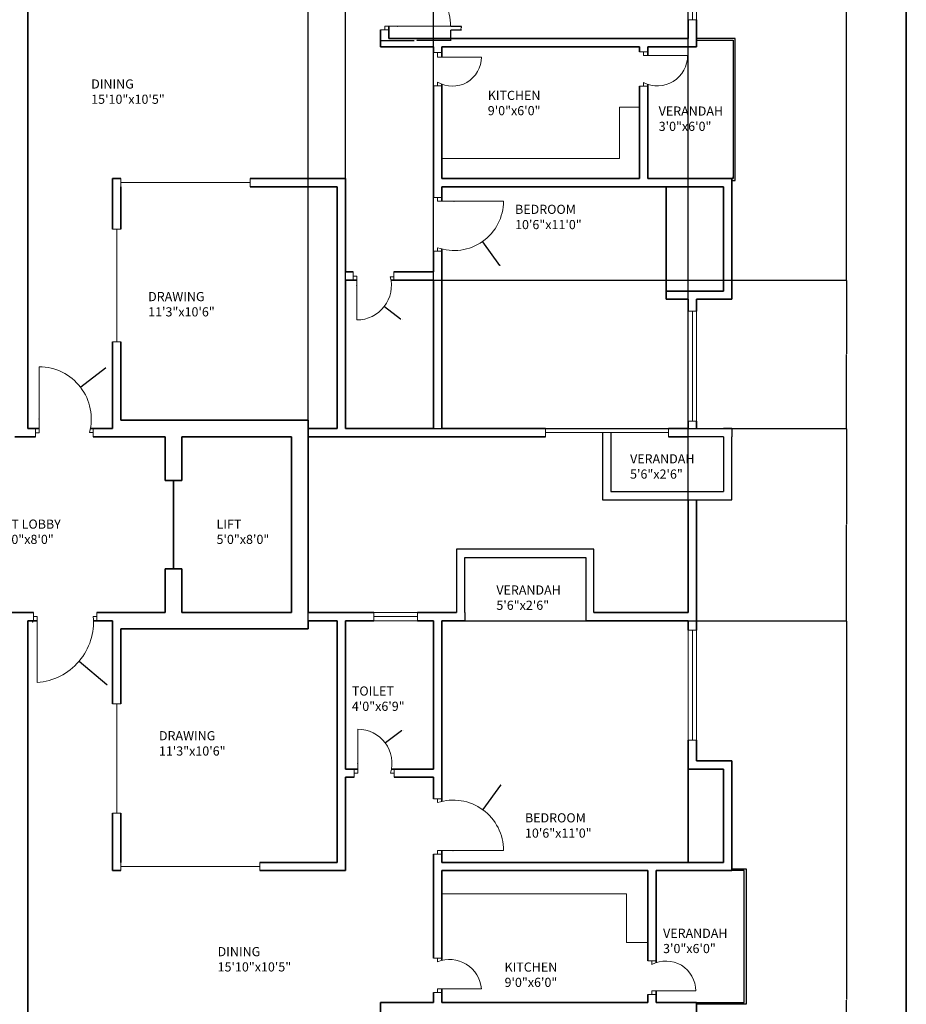
# Model space of a CAD drawing. Units: inches. Extents: x 2154 to 3131, y 1384 to 2688.
# Tile 4 of 5: x 2647 to 3131, y 1828 to 2365. Entities that reach past the tile are written whole.
import ezdxf

# ---------------------------------------------------------------- set-up
doc = ezdxf.new("R2010")
doc.units = ezdxf.units.IN
for name, color, linetype, lineweight in [('A-ANNO-DIMS', 2, 'Continuous', 18), ('A-ANNO-TTLB', 7, 'Continuous', 35), ('A-AREA-IDEN', 7, 'Continuous', 18), ('A-DOOR', 31, 'Continuous', 18), ('A-FLOR-BALC', 130, 'Continuous', 25), ('A-FLOR-EVTR', 7, 'Continuous', 35), ('A-FLOR-FIXT', 8, 'Continuous', 18), ('A-GLAZ', 130, 'Continuous', 18), ('A-WALL', 7, 'Continuous', 35)]:
    doc.layers.add(name, color=color, linetype=linetype, lineweight=lineweight)
doc.styles.get("Standard").update_dxf_attribs({"font": 'arial.ttf'})
doc.dimstyles.get("Standard").update_dxf_attribs({"dimtxt": 0.18, "dimasz": 0.18, "dimexe": 0.18, "dimexo": 0.0625, "dimgap": 0.09, "dimtad": 0, "dimtih": 1, "dimtoh": 1, "dimdec": 4, "dimzin": 0, "dimdsep": 46, "dimtxsty": 'Standard', "dimcen": 0.09, "dimadec": 0, "dimazin": 0, "dimtfac": 1, "dimtdec": 4, "dimtofl": 0, "dimtmove": 0, "dimatfit": 3, "dimfxl": 1, "dimtolj": 1, "dimtzin": 0, "dimarcsym": 0})

# ---------------------------------------------------------------- blocks, each defined once
blk = doc.blocks.new('DOOR-LEAF-24-JAMB-A')
for p, q in [((0, 2.25), (0, 26.25)), ((2, 2.25), (0, 2.25)), ((2, 4.5), (2, 0)), ((2, 0), (2, 2.25))]:
    blk.add_line(p, q)
blk = doc.blocks.new('DOOR-LEAF-36-JAMB-A')
for p, q in [((2, 2.25), (2, 38.25)), ((0, 4.5), (0, 0)), ((0, 0), (0, 2.25)), ((0, 2.25), (2, 2.25))]:
    blk.add_line(p, q)
blk = doc.blocks.new('DOOR-LEAF-24-JAMB-B')
for p, q in [((0, 2), (4.5, 2)), ((4.5, 2), (2.25, 2)), ((2.25, 2), (2.25, 0)), ((2.25, 0), (26.25, 0))]:
    blk.add_line(p, q)
blk = doc.blocks.new('DOOR-LEAF-36-JAMB-B')
for p, q in [((2.25, 0), (2.25, 2)), ((2.25, 2), (38.25, 2)), ((0, 0), (4.5, 0)), ((4.5, 0), (2.25, 0))]:
    blk.add_line(p, q)
blk = doc.blocks.new('WIN-60')
for p, q in [((2.25, 60), (0, 60)), ((0, 60), (4.5, 60)), ((0, 60), (0, 0)), ((2.25, 0), (2.25, 60)), ((4.5, 60), (4.5, 0)), ((0, 0), (4.5, 0)), ((4.5, 0), (2.25, 0))]:
    blk.add_line(p, q)
blk = doc.blocks.new('WIN-24-FRAME-B')
for p, q in [((0, 0), (0, 4.5)), ((0, 4.5), (24, 4.5)), ((24, 2.25), (0, 2.25)), ((0, 2.25), (0, 0)), ((24, 4.5), (24, 0)), ((24, 0), (24, 2.25)), ((24, 0), (0, 0))]:
    blk.add_line(p, q)
blk = doc.blocks.new('*D14')
at = {"layer": 'A-ANNO-DIMS', "color": 0, "lineweight": -2, "transparency": 16777216}
for p, q in [((2844.16, 2359.75), (2844.16, 2353.89)), ((2882.41, 2359.75), (2882.41, 2353.89)), ((2844.34, 2354.07), (2862.56, 2354.07)), ((2882.23, 2354.07), (2864, 2354.07))]:
    blk.add_line(p, q, dxfattribs=at)
at = {"layer": 'A-ANNO-DIMS', "color": 0, "transparency": 16777216}
for points in [[(2844.34, 2354.1), (2844.34, 2354.04), (2844.16, 2354.07)], [(2882.23, 2354.1), (2882.23, 2354.04), (2882.41, 2354.07)]]:
    blk.add_solid(points, dxfattribs=at)
at = {"layer": 'Defpoints', "color": 0, "transparency": 16777216}
for p in [(2844.16, 2359.81), (2882.41, 2359.81), (2882.41, 2354.07)]:
    blk.add_point(p, dxfattribs=at)
at = {"layer": 'A-ANNO-DIMS', "color": 0, "transparency": 16777216, "insert": (2863.28, 2354.07), "char_height": 0.18, "attachment_point": 5}
blk.add_mtext('\\A1;D4 38 TYP.', dxfattribs=at)
blk = doc.blocks.new('*D15')
at = {"layer": 'A-ANNO-DIMS', "color": 0, "lineweight": -2, "transparency": 16777216}
for p, q in [((2882.47, 2361.81), (2888.32, 2361.81)), ((2888.14, 2361.63), (2888.14, 2360.99)), ((2882.47, 2359.81), (2888.32, 2359.81)), ((2888.14, 2359.99), (2888.14, 2360.63))]:
    blk.add_line(p, q, dxfattribs=at)
at = {"layer": 'A-ANNO-DIMS', "color": 0, "transparency": 16777216}
for points in [[(2888.11, 2361.63), (2888.17, 2361.63), (2888.14, 2361.81)], [(2888.11, 2359.99), (2888.17, 2359.99), (2888.14, 2359.81)]]:
    blk.add_solid(points, dxfattribs=at)
at = {"layer": 'Defpoints', "color": 0, "transparency": 16777216}
for p in [(2882.41, 2361.81), (2888.14, 2361.81), (2882.41, 2359.81)]:
    blk.add_point(p, dxfattribs=at)
at = {"layer": 'A-ANNO-DIMS', "color": 0, "transparency": 16777216, "insert": (2888.14, 2360.81), "char_height": 0.18, "attachment_point": 5}
blk.add_mtext('\\A1;2 TYP.', dxfattribs=at)
blk = doc.blocks.new('*D27')
at = {"layer": 'A-ANNO-DIMS', "color": 0, "lineweight": -2, "transparency": 16777216}
for p, q in [((2804.6, 2037.24), (2804.6, 2635.76)), ((2804.78, 2635.58), (2907.91, 2635.58)), ((3011.98, 2635.58), (2908.84, 2635.58)), ((3012.16, 2041.74), (3012.16, 2635.76))]:
    blk.add_line(p, q, dxfattribs=at)
at = {"layer": 'A-ANNO-DIMS', "color": 0, "transparency": 16777216}
for points in [[(2804.78, 2635.61), (2804.78, 2635.55), (2804.6, 2635.58)], [(3011.98, 2635.61), (3011.98, 2635.55), (3012.16, 2635.58)]]:
    blk.add_solid(points, dxfattribs=at)
at = {"layer": 'Defpoints', "color": 0, "transparency": 16777216}
for p in [(3012.16, 2635.58), (3012.16, 2041.68), (2804.6, 2037.18)]:
    blk.add_point(p, dxfattribs=at)
at = {"layer": 'A-ANNO-DIMS', "color": 0, "transparency": 16777216, "insert": (2908.38, 2635.58), "char_height": 0.18, "attachment_point": 5}
blk.add_mtext('\\A1;207.56', dxfattribs=at)
blk = doc.blocks.new('*D30')
at = {"layer": 'A-ANNO-DIMS', "color": 0, "lineweight": -2, "transparency": 16777216}
for p, q in [((3012.22, 2037.18), (3098.74, 2037.18)), ((3098.56, 2037), (3098.56, 1830.36)), ((3098.56, 1623.36), (3098.56, 1830)), ((3016.72, 1623.18), (3098.74, 1623.18))]:
    blk.add_line(p, q, dxfattribs=at)
at = {"layer": 'A-ANNO-DIMS', "color": 0, "transparency": 16777216}
for points in [[(3098.53, 2037), (3098.59, 2037), (3098.56, 2037.18)], [(3098.53, 1623.36), (3098.59, 1623.36), (3098.56, 1623.18)]]:
    blk.add_solid(points, dxfattribs=at)
at = {"layer": 'Defpoints', "color": 0, "transparency": 16777216}
for p in [(3012.16, 2037.18), (3098.56, 2037.18), (3016.66, 1623.18)]:
    blk.add_point(p, dxfattribs=at)
at = {"layer": 'A-ANNO-DIMS', "color": 0, "transparency": 16777216, "insert": (3098.56, 1830.18), "char_height": 0.18, "attachment_point": 5}
blk.add_mtext('\\A1;414', dxfattribs=at)
blk = doc.blocks.new('*D31')
at = {"layer": 'A-ANNO-DIMS', "color": 0, "lineweight": -2, "transparency": 16777216}
for p, q in [((3016.72, 2142.21), (3098.74, 2142.21)), ((3098.56, 2142.03), (3098.56, 2089.87)), ((3098.56, 2037.36), (3098.56, 2089.51)), ((3012.22, 2037.18), (3098.74, 2037.18))]:
    blk.add_line(p, q, dxfattribs=at)
at = {"layer": 'A-ANNO-DIMS', "color": 0, "transparency": 16777216}
for points in [[(3098.53, 2142.03), (3098.59, 2142.03), (3098.56, 2142.21)], [(3098.53, 2037.36), (3098.59, 2037.36), (3098.56, 2037.18)]]:
    blk.add_solid(points, dxfattribs=at)
at = {"layer": 'Defpoints', "color": 0, "transparency": 16777216}
for p in [(3016.66, 2142.21), (3098.56, 2142.21), (3012.16, 2037.18)]:
    blk.add_point(p, dxfattribs=at)
at = {"layer": 'A-ANNO-DIMS', "color": 0, "transparency": 16777216, "insert": (3098.56, 2089.69), "char_height": 0.18, "attachment_point": 5}
blk.add_mtext('\\A1;105.03', dxfattribs=at)
blk = doc.blocks.new('*D32')
at = {"layer": 'A-ANNO-DIMS', "color": 0, "lineweight": -2, "transparency": 16777216}
for p, q in [((2873.1, 2223.18), (3098.74, 2223.18)), ((3098.56, 2223), (3098.56, 2182.86)), ((3098.56, 2142.36), (3098.56, 2182.49)), ((2873.1, 2142.18), (3098.74, 2142.18))]:
    blk.add_line(p, q, dxfattribs=at)
at = {"layer": 'A-ANNO-DIMS', "color": 0, "transparency": 16777216}
for points in [[(3098.53, 2223), (3098.59, 2223), (3098.56, 2223.18)], [(3098.53, 2142.36), (3098.59, 2142.36), (3098.56, 2142.18)]]:
    blk.add_solid(points, dxfattribs=at)
at = {"layer": 'Defpoints', "color": 0, "transparency": 16777216}
for p in [(2873.04, 2223.18), (3098.56, 2223.18), (2873.04, 2142.18)]:
    blk.add_point(p, dxfattribs=at)
at = {"layer": 'A-ANNO-DIMS', "color": 0, "transparency": 16777216, "insert": (3098.56, 2182.68), "char_height": 0.18, "attachment_point": 5}
blk.add_mtext('\\A1;81', dxfattribs=at)
blk = doc.blocks.new('*D33')
at = {"layer": 'A-ANNO-DIMS', "color": 0, "lineweight": -2, "transparency": 16777216}
for p, q in [((3016.72, 2562.18), (3098.74, 2562.18)), ((3098.56, 2562), (3098.56, 2392.86)), ((3098.56, 2223.36), (3098.56, 2392.49)), ((2873.1, 2223.18), (3098.74, 2223.18))]:
    blk.add_line(p, q, dxfattribs=at)
at = {"layer": 'A-ANNO-DIMS', "color": 0, "transparency": 16777216}
for points in [[(3098.53, 2562), (3098.59, 2562), (3098.56, 2562.18)], [(3098.53, 2223.36), (3098.59, 2223.36), (3098.56, 2223.18)]]:
    blk.add_solid(points, dxfattribs=at)
at = {"layer": 'Defpoints', "color": 0, "transparency": 16777216}
for p in [(3016.66, 2562.18), (3098.56, 2562.18), (2873.04, 2223.18)]:
    blk.add_point(p, dxfattribs=at)
at = {"layer": 'A-ANNO-DIMS', "color": 0, "transparency": 16777216, "insert": (3098.56, 2392.68), "char_height": 0.18, "attachment_point": 5}
blk.add_mtext('\\A1;339', dxfattribs=at)
blk = doc.blocks.new('*D34')
at = {"layer": 'A-ANNO-DIMS', "color": 0, "lineweight": -2, "transparency": 16777216}
for p, q in [((2825.04, 2142.24), (2825.04, 2635.76)), ((2825.22, 2635.58), (2848.81, 2635.58)), ((2872.86, 2635.58), (2849.26, 2635.58)), ((2873.04, 2142.24), (2873.04, 2635.76))]:
    blk.add_line(p, q, dxfattribs=at)
at = {"layer": 'A-ANNO-DIMS', "color": 0, "transparency": 16777216}
for points in [[(2825.22, 2635.61), (2825.22, 2635.55), (2825.04, 2635.58)], [(2872.86, 2635.61), (2872.86, 2635.55), (2873.04, 2635.58)]]:
    blk.add_solid(points, dxfattribs=at)
at = {"layer": 'Defpoints', "color": 0, "transparency": 16777216}
for p in [(2873.04, 2635.58), (2825.04, 2142.18), (2873.04, 2142.18)]:
    blk.add_point(p, dxfattribs=at)
at = {"layer": 'A-ANNO-DIMS', "color": 0, "transparency": 16777216, "insert": (2849.04, 2635.58), "char_height": 0.18, "attachment_point": 5}
blk.add_mtext('\\A1;48', dxfattribs=at)
blk = doc.blocks.new('*D35')
at = {"layer": 'A-ANNO-DIMS', "color": 0, "lineweight": -2, "transparency": 16777216}
for p, q in [((2654.17, 2036.55), (2654.35, 2036.55)), ((2654.26, 2036.46), (2654.26, 2036.64)), ((2694.7, 2002.08), (2679.67, 2014.89)), ((2694.88, 2002.08), (2694.7, 2002.08))]:
    blk.add_line(p, q, dxfattribs=at)
at = {"layer": 'A-ANNO-DIMS', "color": 0, "transparency": 16777216}
blk.add_solid([(2679.69, 2014.91), (2679.65, 2014.87), (2679.53, 2015.01)], dxfattribs=at)
at = {"layer": 'Defpoints', "color": 0, "transparency": 16777216}
for p in [(2654.26, 2036.55), (2679.53, 2015.01)]:
    blk.add_point(p, dxfattribs=at)
at = {"layer": 'A-ANNO-DIMS', "color": 0, "transparency": 16777216, "insert": (2695.43, 2002.08), "char_height": 0.18, "attachment_point": 5}
blk.add_mtext('\\A1;R33.214', dxfattribs=at)
blk = doc.blocks.new('*D40')
at = {"layer": 'A-ANNO-DIMS', "color": 0, "lineweight": -2, "transparency": 16777216}
for p, q in [((2882.03, 2398.4), (2871.38, 2384.82)), ((2882.21, 2398.4), (2882.03, 2398.4)), ((2853.25, 2361.81), (2853.43, 2361.81)), ((2853.34, 2361.72), (2853.34, 2361.9))]:
    blk.add_line(p, q, dxfattribs=at)
at = {"layer": 'A-ANNO-DIMS', "color": 0, "transparency": 16777216}
blk.add_solid([(2871.36, 2384.84), (2871.41, 2384.8), (2871.27, 2384.68)], dxfattribs=at)
at = {"layer": 'Defpoints', "color": 0, "transparency": 16777216}
for p in [(2871.27, 2384.68), (2853.34, 2361.81)]:
    blk.add_point(p, dxfattribs=at)
at = {"layer": 'A-ANNO-DIMS', "color": 0, "transparency": 16777216, "insert": (2882.69, 2398.4), "char_height": 0.18, "attachment_point": 5}
blk.add_mtext('\\A1;R29.06', dxfattribs=at)
blk = doc.blocks.new('*D43')
at = {"layer": 'A-ANNO-DIMS', "color": 0, "lineweight": -2, "transparency": 16777216}
for p, q in [((2693.94, 2175.05), (2680.52, 2164.77)), ((2694.12, 2175.05), (2693.94, 2175.05)), ((2657.68, 2147.34), (2657.86, 2147.34)), ((2657.77, 2147.25), (2657.77, 2147.43))]:
    blk.add_line(p, q, dxfattribs=at)
at = {"layer": 'A-ANNO-DIMS', "color": 0, "transparency": 16777216}
blk.add_solid([(2680.5, 2164.79), (2680.54, 2164.75), (2680.38, 2164.66)], dxfattribs=at)
at = {"layer": 'Defpoints', "color": 0, "transparency": 16777216}
for p in [(2680.38, 2164.66), (2657.77, 2147.34)]:
    blk.add_point(p, dxfattribs=at)
at = {"layer": 'A-ANNO-DIMS', "color": 0, "transparency": 16777216, "insert": (2694.6, 2175.05), "char_height": 0.18, "attachment_point": 5}
blk.add_mtext('\\A1;R28.48', dxfattribs=at)
blk = doc.blocks.new('*D47')
at = {"layer": 'A-ANNO-DIMS', "color": 0, "lineweight": -2, "transparency": 16777216}
for p, q in [((2909.69, 1947.29), (2900.06, 1934.08)), ((2909.87, 1947.29), (2909.69, 1947.29)), ((2883.64, 1911.66), (2883.82, 1911.66)), ((2883.73, 1911.57), (2883.73, 1911.75))]:
    blk.add_line(p, q, dxfattribs=at)
at = {"layer": 'A-ANNO-DIMS', "color": 0, "transparency": 16777216}
blk.add_solid([(2900.04, 1934.1), (2900.09, 1934.06), (2899.96, 1933.93)], dxfattribs=at)
at = {"layer": 'Defpoints', "color": 0, "transparency": 16777216}
for p in [(2899.96, 1933.93), (2883.73, 1911.66)]:
    blk.add_point(p, dxfattribs=at)
at = {"layer": 'A-ANNO-DIMS', "color": 0, "transparency": 16777216, "insert": (2910.42, 1947.29), "char_height": 0.18, "attachment_point": 5}
blk.add_mtext('\\A1;R27.553', dxfattribs=at)
blk = doc.blocks.new('*D49')
at = {"layer": 'A-ANNO-DIMS', "color": 0, "lineweight": -2, "transparency": 16777216}
for p, q in [((2884.2, 2266.37), (2884.38, 2266.37)), ((2884.29, 2266.28), (2884.29, 2266.46)), ((2909.23, 2231.09), (2899.98, 2244.17)), ((2909.41, 2231.09), (2909.23, 2231.09))]:
    blk.add_line(p, q, dxfattribs=at)
at = {"layer": 'A-ANNO-DIMS', "color": 0, "transparency": 16777216}
blk.add_solid([(2900, 2244.19), (2899.95, 2244.16), (2899.88, 2244.32)], dxfattribs=at)
at = {"layer": 'Defpoints', "color": 0, "transparency": 16777216}
for p in [(2884.29, 2266.37), (2899.88, 2244.32)]:
    blk.add_point(p, dxfattribs=at)
at = {"layer": 'A-ANNO-DIMS', "color": 0, "transparency": 16777216, "insert": (2909.71, 2231.09), "char_height": 0.18, "attachment_point": 5}
blk.add_mtext('\\A1;R27', dxfattribs=at)
blk = doc.blocks.new('*D59')
at = {"layer": 'A-ANNO-DIMS', "color": 0, "lineweight": -2, "transparency": 16777216}
for p, q in [((2831.18, 2220.22), (2831.36, 2220.22)), ((2831.27, 2220.13), (2831.27, 2220.31)), ((2855.11, 2201.9), (2846.31, 2208.66)), ((2855.29, 2201.9), (2855.11, 2201.9))]:
    blk.add_line(p, q, dxfattribs=at)
at = {"layer": 'A-ANNO-DIMS', "color": 0, "transparency": 16777216}
blk.add_solid([(2846.33, 2208.68), (2846.29, 2208.63), (2846.17, 2208.77)], dxfattribs=at)
at = {"layer": 'Defpoints', "color": 0, "transparency": 16777216}
for p in [(2831.27, 2220.22), (2846.17, 2208.77)]:
    blk.add_point(p, dxfattribs=at)
at = {"layer": 'A-ANNO-DIMS', "color": 0, "transparency": 16777216, "insert": (2855.84, 2201.9), "char_height": 0.18, "attachment_point": 5}
blk.add_mtext('\\A1;R18.793', dxfattribs=at)
blk = doc.blocks.new('*D60')
at = {"layer": 'A-ANNO-DIMS', "color": 0, "lineweight": -2, "transparency": 16777216}
for p, q in [((2855.66, 1977.05), (2846.84, 1970.51)), ((2855.84, 1977.05), (2855.66, 1977.05)), ((2831.67, 1959.34), (2831.85, 1959.34)), ((2831.76, 1959.25), (2831.76, 1959.43))]:
    blk.add_line(p, q, dxfattribs=at)
at = {"layer": 'A-ANNO-DIMS', "color": 0, "transparency": 16777216}
blk.add_solid([(2846.82, 1970.54), (2846.86, 1970.49), (2846.7, 1970.4)], dxfattribs=at)
at = {"layer": 'Defpoints', "color": 0, "transparency": 16777216}
for p in [(2846.7, 1970.4), (2831.76, 1959.34)]:
    blk.add_point(p, dxfattribs=at)
at = {"layer": 'A-ANNO-DIMS', "color": 0, "transparency": 16777216, "insert": (2856.32, 1977.05), "char_height": 0.18, "attachment_point": 5}
blk.add_mtext('\\A1;R18.59', dxfattribs=at)

msp = doc.modelspace()

# ---------------------------------------------------------------- linework, layer by layer
at = {"layer": 'A-ANNO-TTLB'}
msp.add_lwpolyline([(2154.1953, 2688.4009), (3131.1627, 2688.4009), (3131.1627, 1383.7377), (2154.1953, 1383.7377)], close=True, dxfattribs=at)
at = {"layer": 'A-DOOR'}
for p, q in [((2873.0368, 2347.5192), (2877.5368, 2347.5192)), ((2877.5368, 2347.5192), (2875.2868, 2347.5192)), ((2875.2868, 2347.5192), (2875.2868, 2347.0346)), ((2875.2868, 2347.0346), (2875.2868, 2345.0346)), ((2875.2868, 2345.0346), (2899.2868, 2345.0346)), ((2873.0368, 2329.273), (2877.5368, 2329.273)), ((2875.2868, 2329.273), (2875.2868, 2331.273)), ((2877.5368, 2329.273), (2875.2868, 2329.273)), ((2985.5368, 2329.0685), (2990.0368, 2329.0685)), ((2987.7868, 2329.0685), (2987.7868, 2331.0685)), ((2990.0368, 2329.0685), (2987.7868, 2329.0685)), ((2873.0368, 2238.9097), (2877.5368, 2238.9097)), ((2875.2868, 2238.9097), (2875.2868, 2240.9097)), ((2877.5368, 2238.9097), (2875.2868, 2238.9097)), ((2851.4271, 2226.9339), (2851.4271, 2227.6767)), ((2851.4271, 2227.6767), (2851.4271, 2225.0553)), ((2851.4271, 2223.1767), (2851.4271, 2226.9339)), ((2851.4271, 2225.0553), (2849.4271, 2225.0553)), ((2657.7665, 2139.8207), (2657.7665, 2175.8207)), ((2655.7665, 2142.1767), (2655.7665, 2137.6767)), ((2687.2664, 2142.1767), (2687.2664, 2137.6767)), ((2655.7665, 2137.6767), (2655.7665, 2139.8207)), ((2655.7665, 2139.8207), (2655.7665, 2139.8207)), ((2655.7665, 2139.8207), (2657.7665, 2139.8207)), ((2687.2664, 2139.9267), (2685.2664, 2139.9267)), ((2687.2664, 2137.6767), (2687.2664, 2139.9267)), ((2689.347, 2039.4267), (2687.347, 2039.4267)), ((2689.347, 2037.1767), (2689.347, 2041.6767)), ((2689.347, 2041.6767), (2689.347, 2039.4267)), ((2851.5443, 1953.9267), (2849.5443, 1953.9267)), ((2851.5443, 1956.1767), (2851.5443, 1951.6767)), ((2851.5443, 1951.6767), (2851.5443, 1953.9267)), ((2873.0368, 1939.8885), (2877.5368, 1939.8885)), ((2877.5368, 1939.8885), (2875.2868, 1939.8885)), ((2875.2868, 1939.8885), (2875.2868, 1937.8885)), ((2873.0368, 1852.9368), (2877.5368, 1852.9368)), ((2877.5368, 1852.9368), (2875.2868, 1852.9368)), ((2875.2868, 1852.9368), (2875.2868, 1850.9368)), ((2994.5368, 1851.4405), (2990.0368, 1851.4405)), ((2990.0368, 1851.4405), (2992.2868, 1851.4405)), ((2992.2868, 1851.4405), (2992.2868, 1849.4405))]:
    msp.add_line(p, q, dxfattribs=at)
for centre, radius, start, end in [((2853.3445, 2361.81), 29.0615, 360, 103.812872), ((2883.3414, 2345.0346), 15.9454, 239.659886, 360), ((2995.242, 2345.8384), 16.5448, 243.217314, 360), ((2884.2868, 2266.3656), 27, 250.528926, 0), ((2831.267, 2220.2196), 18.7929, 270, 14.910859), ((2657.7665, 2147.3392), 28.4815, 344.914708, 90), ((2654.2571, 2036.5539), 33.2144, 274.152608, 4.961828), ((2831.7604, 1959.3378), 18.5889, 343.076683, 90), ((2883.734, 1911.6624), 27.5528, 0, 107.853291), ((2881.7142, 1834.496), 17.6525, 5.452702, 111.352336), ((2999.9165, 1834.9568), 16.3704, 360, 117.779129)]:
    msp.add_arc(centre, radius, start, end, dxfattribs=at)
at = {"layer": 'A-FLOR-BALC'}
for p, q in [((3037.656, 2355.1767), (3016.656, 2355.1767)), ((3016.656, 2355.1767), (3016.656, 2354.1767)), ((3016.656, 2354.1767), (3036.656, 2354.1767)), ((3036.656, 2354.1767), (3036.656, 2278.6767)), ((3037.656, 2277.6767), (3037.656, 2355.1767)), ((3035.8703, 2278.6767), (3036.656, 2278.6767)), ((3036.656, 2278.6767), (3035.8703, 2278.6767)), ((3035.8703, 2277.6767), (3037.656, 2277.6767)), ((3036.656, 2278.6767), (3036.656, 2279.6767)), ((3016.656, 2142.208), (3035.8703, 2142.208)), ((3035.8703, 2142.208), (3031.3703, 2142.208)), ((3035.8703, 2142.208), (3035.8703, 2137.6767)), ((2965.3703, 2139.9267), (2965.3703, 2107.6767)), ((2969.8703, 2139.9267), (2969.8703, 2107.6767)), ((3031.3703, 2137.6767), (3001.4145, 2137.6767)), ((3031.3703, 2137.6767), (3031.3703, 2107.6767)), ((3035.8703, 2107.6767), (3035.8703, 2137.6767)), ((3035.8703, 2103.1767), (3035.8703, 2108.2932)), ((2965.3703, 2107.6767), (2965.3703, 2103.1767)), ((2965.3703, 2103.1767), (3035.8703, 2103.1767)), ((2969.8703, 2107.6767), (3031.3703, 2107.6767)), ((2890.1344, 2076.1767), (2885.6344, 2076.1767)), ((2885.6344, 2076.1767), (2885.6344, 2041.6767)), ((2960.6344, 2076.1767), (2890.1344, 2076.1767)), ((2960.6344, 2071.6767), (2960.6344, 2076.1767)), ((2890.1344, 2041.6767), (2890.1344, 2071.6767)), ((2890.1344, 2071.6767), (2956.1344, 2071.6767)), ((2956.1344, 2071.6767), (2956.1344, 2041.6767)), ((2960.6344, 2041.6767), (2960.6344, 2071.6767)), ((2890.1344, 2041.6767), (2890.1344, 2037.1767)), ((2956.1344, 2041.6767), (2956.1344, 2037.1767)), ((2890.1344, 2037.1767), (2956.1344, 2037.1767)), ((3035.8703, 1900.6767), (3035.8703, 1901.6767)), ((3035.8703, 1901.6767), (3042.656, 1901.6767)), ((3042.656, 1900.6767), (3035.8703, 1900.6767)), ((3042.656, 1901.6767), (3043.656, 1901.6767)), ((3042.656, 1828.6767), (3042.656, 1900.6767)), ((3043.656, 1901.6767), (3043.656, 1827.6767)), ((3016.656, 1828.6767), (3018.656, 1828.6767)), ((3018.656, 1828.6767), (3042.656, 1828.6767)), ((3043.656, 1829.2556), (3043.656, 1828.2556)), ((3043.656, 1827.6767), (3016.656, 1827.6767))]:
    msp.add_line(p, q, dxfattribs=at)
at = {"layer": 'A-FLOR-EVTR'}
for p, q in [((2804.5995, 2146.6767), (2702.4352, 2146.6767)), ((2804.5995, 2142.1767), (2804.5995, 2146.6767)), ((2804.5995, 2041.6767), (2804.5995, 2142.1767)), ((2726.5995, 2137.6767), (2726.5995, 2113.7762)), ((2735.5995, 2137.6767), (2795.5995, 2137.6767)), ((2735.5995, 2137.6767), (2795.5995, 2137.6767)), ((2735.5995, 2113.7762), (2735.5995, 2137.6767)), ((2795.5995, 2137.6767), (2795.5995, 2041.6767)), ((2726.5995, 2113.7762), (2735.5995, 2113.7762)), ((2731.0995, 2113.7762), (2731.0995, 2065.442)), ((2726.5995, 2065.442), (2735.5995, 2065.442)), ((2726.5995, 2065.442), (2726.5995, 2041.6767)), ((2735.5995, 2041.6767), (2735.5995, 2065.442)), ((2735.5995, 2041.6767), (2795.5995, 2041.6767)), ((2804.5995, 2032.6767), (2702.3466, 2032.6767)), ((2804.5995, 2037.1767), (2804.5995, 2032.6767))]:
    msp.add_line(p, q, dxfattribs=at)
at = {"layer": 'A-FLOR-FIXT'}
for p, q in [((2985.5368, 2317.5781), (2974.5593, 2317.5781)), ((2974.5593, 2317.5781), (2974.5593, 2289.5283)), ((2974.5593, 2289.5283), (2877.5368, 2289.5283)), ((2978.3352, 1888.0055), (2877.5368, 1888.0055)), ((2978.3352, 1861.5173), (2978.3352, 1888.0055)), ((2990.0368, 1861.5173), (2978.3352, 1861.5173))]:
    msp.add_line(p, q, dxfattribs=at)
at = {"layer": 'A-GLAZ'}
for p, q in [((2702.4352, 2274.1767), (2702.4352, 2278.6767)), ((2702.4352, 2278.6767), (2702.4352, 2276.4267)), ((2702.4352, 2276.4267), (2772.9337, 2276.4267)), ((2772.9337, 2274.1767), (2772.9337, 2278.6767)), ((2772.9337, 2278.6767), (2772.9337, 2274.1767)), ((2697.8466, 2250.9284), (2702.4352, 2250.9284)), ((2702.4352, 2250.9284), (2700.1409, 2250.9284)), ((2700.1409, 2250.9284), (2700.1409, 2189.4501)), ((2700.1409, 2189.4501), (2697.8466, 2189.4501)), ((2697.8466, 2189.4501), (2702.4352, 2189.4501)), ((2934.2505, 2142.1767), (2934.2505, 2137.6767)), ((3001.4145, 2139.9267), (3001.4145, 2142.1767)), ((3001.4145, 2142.1767), (3001.4145, 2137.6767)), ((2934.2505, 2137.6767), (2934.2505, 2139.9267)), ((2934.2505, 2139.9267), (3001.4145, 2139.9267)), ((3016.656, 2031.9267), (3012.156, 2031.9267)), ((3012.156, 1971.9781), (3012.156, 2031.9267)), ((3014.406, 1971.9781), (3014.406, 2031.9781)), ((3014.406, 2031.9781), (3016.656, 2031.9267)), ((3016.656, 2031.9267), (3016.656, 2031.9267)), ((3016.656, 2031.9267), (3016.656, 1971.9781)), ((2700.0966, 1991.7924), (2697.8466, 1991.7924)), ((2697.8466, 1991.7924), (2702.3466, 1991.7924)), ((2700.0966, 1932.0522), (2700.0966, 1991.7924)), ((3012.156, 1971.9781), (3016.656, 1971.9781)), ((3016.656, 1971.9781), (3014.406, 1971.9781)), ((2697.8466, 1932.0522), (2702.3466, 1932.0522)), ((2702.3466, 1932.0522), (2700.0966, 1932.0522)), ((2702.3466, 1902.9267), (2702.3466, 1905.1767)), ((2702.3466, 1905.1767), (2702.3466, 1900.6767)), ((2778.1809, 1905.1767), (2778.1809, 1900.6767)), ((2778.1809, 1902.9267), (2702.3466, 1902.9267)), ((2778.1809, 1900.6767), (2778.1809, 1902.9267))]:
    msp.add_line(p, q, dxfattribs=at)
at = {"layer": 'A-WALL'}
for p, q in [((2651.656, 2400.1767), (2651.656, 2142.1767)), ((2848.656, 2361.81), (2848.656, 2355.1767)), ((3012.156, 2365.4173), (3012.156, 2355.1767)), ((3016.656, 2365.4173), (3016.656, 2350.6767)), ((2844.156, 2359.81), (2844.156, 2350.6767)), ((2844.156, 2350.6767), (2873.0368, 2350.6767)), ((2848.656, 2355.1767), (3012.156, 2355.1767)), ((2873.0368, 2350.6767), (2873.0368, 2347.5192)), ((2877.5368, 2345.0346), (2877.5368, 2350.6767)), ((2877.5368, 2350.6767), (2985.5368, 2350.6767)), ((2985.5368, 2347.8384), (2985.5368, 2350.6767)), ((2990.0368, 2350.6767), (2990.0368, 2350.6767)), ((2990.0368, 2350.6767), (2990.0368, 2345.8384)), ((2990.0368, 2350.6767), (3016.656, 2350.6767)), ((2873.0368, 2329.273), (2873.0368, 2278.6767)), ((2877.5368, 2278.6767), (2877.5368, 2330.1832)), ((2985.5368, 2278.6767), (2985.5368, 2329.0685)), ((2990.0368, 2330.1338), (2990.0368, 2278.6767)), ((2697.8466, 2278.6767), (2697.8466, 2250.9284)), ((2697.8466, 2278.6767), (2702.4352, 2278.6767)), ((2702.4352, 2278.6767), (2697.8466, 2278.6767)), ((2825.0368, 2278.6767), (2772.9337, 2278.6767)), ((2772.9337, 2278.6767), (2825.0368, 2278.6767)), ((2825.0368, 2227.6767), (2825.0368, 2278.6767)), ((2873.0368, 2268.3656), (2873.0368, 2278.6767)), ((2877.5368, 2278.6767), (2985.5368, 2278.6767)), ((2985.5368, 2278.6767), (2877.5368, 2278.6767)), ((2990.0368, 2278.6767), (3016.656, 2278.6767)), ((3035.8703, 2278.6767), (2990.0368, 2278.6767)), ((2990.0368, 2278.6767), (3035.8703, 2278.6767)), ((3035.8703, 2278.6767), (3016.656, 2278.6767)), ((3035.8703, 2278.6767), (3035.8703, 2277.6767)), ((3035.8703, 2277.6767), (3035.8703, 2212.7046)), ((2702.4352, 2274.1767), (2702.4352, 2250.9284)), ((2772.9337, 2274.1767), (2820.5368, 2274.1767)), ((2820.5368, 2142.1767), (2820.5368, 2274.1767)), ((2877.5368, 2274.1767), (2877.5368, 2266.3656)), ((2877.5368, 2274.1767), (3031.3703, 2274.1767)), ((3000.156, 2217.2046), (3000.156, 2274.1767)), ((3012.156, 2274.1767), (3031.3703, 2274.1767)), ((3031.3703, 2274.1767), (3031.3703, 2217.2046)), ((2873.0368, 2227.6767), (2873.0368, 2238.9097)), ((2877.5368, 2240.2229), (2877.5368, 2142.1767)), ((2825.0368, 2227.6767), (2829.267, 2227.6767)), ((2851.4271, 2227.6767), (2873.0368, 2227.6767)), ((2825.0368, 2142.1767), (2825.0368, 2223.1767)), ((2825.0368, 2223.1767), (2831.267, 2223.1767)), ((2849.8258, 2223.1767), (2873.0368, 2223.1767)), ((2873.0368, 2142.1767), (2873.0368, 2223.1767)), ((3000.156, 2212.7046), (3000.156, 2217.2046)), ((3000.156, 2217.2046), (3012.156, 2217.2046)), ((3031.3703, 2217.2046), (3012.156, 2217.2046)), ((3012.156, 2212.7046), (3000.156, 2212.7046)), ((3012.156, 2212.7046), (3012.156, 2206.1679)), ((3035.8703, 2212.7046), (3016.656, 2212.7046)), ((3016.656, 2212.7046), (3016.656, 2206.1679)), ((2697.8466, 2189.4501), (2697.8466, 2142.1767)), ((2702.4352, 2189.4501), (2702.4352, 2146.6767)), ((3012.156, 2146.1679), (3012.156, 2142.1767)), ((3016.656, 2146.1679), (3016.656, 2142.208)), ((2651.656, 2142.1767), (2657.7665, 2142.1767)), ((2685.7761, 2142.1767), (2697.8466, 2142.1767)), ((2804.5995, 2142.1767), (2820.5368, 2142.1767)), ((2825.0368, 2142.1767), (2873.0368, 2142.1767)), ((2877.5368, 2142.1767), (2934.2505, 2142.1767)), ((3001.4145, 2142.1767), (3012.156, 2142.1767)), ((2644.4666, 2137.6767), (2655.7665, 2137.6767)), ((2687.2664, 2137.6767), (2726.5995, 2137.6767)), ((2804.5995, 2137.6767), (2934.2505, 2137.6767)), ((3001.4145, 2137.6767), (3012.156, 2137.6767)), ((3012.156, 2103.1767), (3012.156, 2041.6767)), ((3016.656, 2103.1767), (3016.656, 2031.9267)), ((2642.2555, 2041.6767), (2654.6623, 2041.6767)), ((2689.347, 2041.6767), (2726.5995, 2041.6767)), ((2804.5995, 2041.6767), (2840.3947, 2041.6767)), ((2864.3947, 2041.6767), (2885.6344, 2041.6767)), ((2960.6344, 2041.6767), (3012.156, 2041.6767)), ((2651.656, 2037.1767), (2651.656, 1782.1799)), ((2651.656, 2037.1767), (2656.6623, 2037.1767)), ((2687.4657, 2037.1767), (2697.8466, 2037.1767)), ((2697.8466, 2037.1767), (2697.8466, 1991.7924)), ((2702.3466, 1991.7924), (2702.3466, 2032.6767)), ((2804.5995, 2037.1767), (2820.5368, 2037.1767)), ((2820.5368, 2037.1767), (2820.5368, 1905.1767)), ((2825.0368, 2037.1767), (2825.0368, 1956.1767)), ((2825.0368, 2037.1767), (2840.3947, 2037.1767)), ((2864.3947, 2037.1767), (2873.0368, 2037.1767)), ((2873.0368, 2037.1767), (2873.0368, 1956.1767)), ((2877.5368, 2037.1767), (2890.1344, 2037.1767)), ((2877.5368, 1938.5093), (2877.5368, 2037.1767)), ((2890.1344, 2037.1767), (2886.156, 2037.1767)), ((3012.156, 2037.1767), (2956.1344, 2037.1767)), ((2956.1344, 2037.1767), (3012.156, 2037.1767)), ((3012.156, 2037.1767), (3012.156, 2031.9267)), ((3012.156, 1971.9781), (3012.156, 1956.1767)), ((3016.656, 1971.9781), (3016.656, 1960.6767)), ((3012.156, 1960.6767), (3012.156, 1956.1767)), ((3035.8703, 1960.6767), (3016.656, 1960.6767)), ((3035.8703, 1960.6767), (3035.8703, 1900.6767)), ((2825.0368, 1956.1767), (2831.7604, 1956.1767)), ((2850.0785, 1956.1767), (2873.0368, 1956.1767)), ((3012.156, 1956.1767), (3031.3703, 1956.1767)), ((3012.156, 1956.1767), (3012.156, 1908.6107)), ((3031.3703, 1956.1767), (3031.3703, 1905.1767)), ((2825.0368, 1951.6767), (2829.7604, 1951.6767)), ((2825.0368, 1951.6767), (2825.0368, 1900.6767)), ((2851.5443, 1951.6767), (2873.0368, 1951.6767)), ((2873.0368, 1951.6767), (2873.0368, 1939.8885)), ((2697.8466, 1932.0522), (2697.8466, 1900.6767)), ((2702.3466, 1905.1767), (2702.3466, 1932.0522)), ((2873.0368, 1909.6624), (2873.0368, 1900.6767)), ((2877.5368, 1905.1767), (2877.5368, 1911.6624)), ((2778.1809, 1905.1767), (2820.5368, 1905.1767)), ((2877.5368, 1905.1767), (3012.156, 1905.1767)), ((3012.156, 1908.6107), (3012.156, 1905.1767)), ((3031.3703, 1905.1767), (3012.156, 1905.1767)), ((2697.8466, 1900.6767), (2702.3466, 1900.6767)), ((2778.1809, 1900.6767), (2825.0368, 1900.6767)), ((2873.0368, 1900.6767), (2873.0368, 1852.9368)), ((2877.5368, 1900.6767), (2990.0368, 1900.6767)), ((2877.5368, 1851.6471), (2877.5368, 1900.6767)), ((2990.0368, 1900.6767), (2990.0368, 1851.4405)), ((2994.5368, 1900.6767), (2994.5368, 1850.418)), ((2994.5368, 1900.6767), (3012.156, 1900.6767)), ((3012.156, 1900.6767), (3035.8703, 1900.6767)), ((2873.0368, 1834.1734), (2873.0368, 1828.6767)), ((2877.5368, 1828.6767), (2877.5368, 1836.1734)), ((2994.5368, 1834.9568), (2994.5368, 1828.6767)), ((2848.656, 1828.6767), (2844.156, 1828.6767)), ((2844.156, 1828.6767), (2844.156, 1818.3686)), ((2873.0368, 1828.6767), (2848.656, 1828.6767)), ((2877.5368, 1828.6767), (2990.0368, 1828.6767)), ((2990.0368, 1832.9568), (2990.0368, 1828.6767)), ((2994.5368, 1828.6767), (3016.656, 1828.6767)), ((3016.656, 1828.6767), (3016.656, 1746.1767))]:
    msp.add_line(p, q, dxfattribs=at)

# ---------------------------------------------------------------- block references
at = {"layer": 'A-DOOR'}
for name, p in [('DOOR-LEAF-36-JAMB-B', (2844.156, 2359.81)), ('DOOR-LEAF-24-JAMB-B', (2985.5368, 2345.8384))]:
    msp.add_blockref(name, p, dxfattribs=at)
at = {"layer": 'A-DOOR', "extrusion": (0, 0, -1), "zscale": -1}
for name, p, rotation in [('DOOR-LEAF-36-JAMB-B', (-2873.0368, 2268.3656), 180), ('DOOR-LEAF-24-JAMB-B', (-2831.267, 2227.6767), 269.9999999999999), ('DOOR-LEAF-36-JAMB-A', (-2654.6623, 2041.6767), 180), ('DOOR-LEAF-36-JAMB-A', (-2873.0368, 1909.6624), 90.00000000000043), ('DOOR-LEAF-24-JAMB-B', (-2873.0368, 1836.1734), 180), ('DOOR-LEAF-24-JAMB-B', (-2990.0368, 1834.9568), 180)]:
    msp.add_blockref(name, p, dxfattribs=dict(at, rotation=rotation))
msp.add_blockref('DOOR-LEAF-24-JAMB-A', (-2831.7604, 1951.6767), dxfattribs=at)
at = {"layer": 'A-GLAZ'}
for name, p in [('WIN-60', (3012.156, 2365.4173)), ('WIN-24-FRAME-B', (2840.3947, 2037.1767))]:
    msp.add_blockref(name, p, dxfattribs=at)
at = {"layer": 'A-GLAZ', "rotation": 180}
msp.add_blockref('WIN-60', (3016.656, 2206.1679), dxfattribs=at)

# ---------------------------------------------------------------- texts
at = {"layer": 'A-AREA-IDEN', "char_height": 5, "attachment_point": 1}
for s, width, insert in [('DINING\\P15\'10"x10\'5"', 240.932067, (2686.1852, 2332.8126)), ('KITCHEN\\P9\'0"x6\'0"', 178.387745, (2902.6811, 2326.5765)), ('VERANDAH\\P3\'0"x6\'0"', 116.935568, (2995.9844, 2318.0106)), ('BEDROOM\\P10\'6"x11\'0"', 156.837412, (2917.592, 2264.3544)), ('DRAWING\\P11\'3"x10\'6"', 194.403518, (2717.2754, 2216.6909)), ('VERANDAH\\P5\'6"x2\'6"', 99.773931, (2980.3645, 2128.0966)), ('LIFT LOBBY\\P11\'0"x8\'0"', 149.609015, (2633.1561, 2092.4357)), ('LIFT\\P5\'0"x8\'0"', 110.246252, (2754.6166, 2092.4357)), ('VERANDAH\\P5\'6"x2\'6"', 146.107868, (2907.3816, 2056.4474)), ('TOILET\\P4\'0"x6\'9"', 146.290484, (2828.4984, 2001.2742)), ('DRAWING\\P11\'3"x10\'6"', 212.345341, (2723.1727, 1976.8531)), ('BEDROOM\\P10\'6"x11\'0"', 140.584633, (2923.005, 1932.0154)), ('VERANDAH\\P3\'0"x6\'0"', 232.123183, (2998.3783, 1868.9714)), ('DINING\\P15\'10"x10\'5"', 244.835501, (2755.2094, 1858.9377)), ('KITCHEN\\P9\'0"x6\'0"', 98.646246, (2911.8466, 1850.5034))]:
    msp.add_mtext_dynamic_manual_height_columns(s, width=width, gutter_width=12.5, heights=[0], dxfattribs=dict(at, insert=insert))

# ---------------------------------------------------------------- dimensions: what is measured, and where the dimension line sits
at = {"layer": 'A-ANNO-DIMS'}
for base, p1, p2, override, picture, middle in [((3012.156, 2635.5767), (2804.5995, 2037.1767), (3012.156, 2041.6767), {"dimdec": 2, "dimlfac": 1, "dimrnd": 0, "dimzin": 0, "dimdsep": 46, "dimlunit": 2}, '*D27', (2908.3778, 2635.5767)), ((2873.0368, 2635.5767), (2825.0368, 2142.1767), (2873.0368, 2142.1767), {"dimdec": 0, "dimlfac": 1, "dimrnd": 0, "dimzin": 0, "dimdsep": 46, "dimlunit": 2}, '*D34', (2849.0368, 2635.5767))]:
    dim = msp.add_linear_dim(base=base, p1=p1, p2=p2, dimstyle='Standard', override=override, dxfattribs=at)
    dim.commit()
    dim.dimension.update_dxf_attribs({"geometry": picture, "text_midpoint": middle})
for base, p1, p2, override, picture, middle in [((3098.556, 2562.1767), (2873.0368, 2223.1767), (3016.656, 2562.1767), {"dimdec": 0, "dimlfac": 1, "dimrnd": 0, "dimzin": 0, "dimdsep": 46, "dimlunit": 2}, '*D33', (3098.556, 2392.6767)), ((3098.556, 2223.1767), (2873.0368, 2142.1767), (2873.0368, 2223.1767), {"dimdec": 0, "dimlfac": 1, "dimrnd": 0, "dimzin": 0, "dimdsep": 46, "dimlunit": 2}, '*D32', (3098.556, 2182.6767)), ((3098.556, 2142.208), (3012.156, 2037.1767), (3016.656, 2142.208), {"dimdec": 2, "dimlfac": 1, "dimrnd": 0, "dimzin": 0, "dimdsep": 46, "dimlunit": 2}, '*D31', (3098.556, 2089.6924)), ((3098.556, 2037.1767), (3016.656, 1623.1767), (3012.156, 2037.1767), {"dimdec": 0, "dimlfac": 1, "dimrnd": 0, "dimzin": 0, "dimdsep": 46, "dimlunit": 2}, '*D30', (3098.556, 1830.1767))]:
    dim = msp.add_linear_dim(base=base, p1=p1, p2=p2, angle=90, dimstyle='Standard', override=override, dxfattribs=at)
    dim.commit()
    dim.dimension.update_dxf_attribs({"geometry": picture, "text_midpoint": middle})
for center, mpoint, override, picture, middle in [((2853.3445, 2361.81), (2871.2737, 2384.6817), {"dimdec": 2, "dimlfac": 1, "dimrnd": 0, "dimzin": 0, "dimdsep": 46, "dimlunit": 2}, '*D40', (2882.6911, 2398.4047)), ((2884.2868, 2266.3656), (2899.875, 2244.32), {"dimdec": 0, "dimlfac": 1, "dimrnd": 0, "dimzin": 0, "dimdsep": 46, "dimlunit": 2}, '*D49', (2909.713, 2231.0926)), ((2831.267, 2220.2196), (2846.1675, 2208.7676), {"dimdec": 3, "dimlfac": 1, "dimrnd": 0, "dimzin": 0, "dimdsep": 46, "dimlunit": 2}, '*D59', (2855.8376, 2201.8964)), ((2657.7665, 2147.3392), (2680.375, 2164.661), {"dimdec": 2, "dimlfac": 1, "dimrnd": 0, "dimzin": 0, "dimdsep": 46, "dimlunit": 2}, '*D43', (2694.6002, 2175.0541)), ((2654.2571, 2036.5539), (2679.535, 2015.008), {"dimdec": 3, "dimlfac": 1, "dimrnd": 0, "dimzin": 0, "dimdsep": 46, "dimlunit": 2}, '*D35', (2695.4311, 2002.0805)), ((2831.7604, 1959.3378), (2846.6958, 1970.4049), {"dimdec": 2, "dimlfac": 1, "dimrnd": 0, "dimzin": 0, "dimdsep": 46, "dimlunit": 2}, '*D60', (2856.3171, 1977.0451)), ((2883.734, 1911.6624), (2899.9581, 1933.9321), {"dimdec": 3, "dimlfac": 1, "dimrnd": 0, "dimzin": 0, "dimdsep": 46, "dimlunit": 2}, '*D47', (2910.4223, 1947.2939))]:
    dim = msp.add_radius_dim(center=center, mpoint=mpoint, dimstyle='Standard', override=override, dxfattribs=at)
    dim.commit()
    dim.dimension.update_dxf_attribs({"geometry": picture, "text_midpoint": middle, "dimtype": 164})
dim = msp.add_linear_dim(base=(2888.1435, 2361.81), p1=(2882.406, 2359.81), p2=(2882.406, 2361.81), angle=90, text='<> TYP.', dimstyle='Standard', override={"dimdec": 0, "dimlfac": 1, "dimrnd": 0, "dimzin": 0, "dimdsep": 46, "dimlunit": 2}, dxfattribs=at)
dim.commit()
dim.dimension.update_dxf_attribs({"geometry": '*D15', "text_midpoint": (2888.1435, 2360.81)})
dim = msp.add_linear_dim(base=(2882.406, 2354.0725), p1=(2844.156, 2359.81), p2=(2882.406, 2359.81), text='D4 <> TYP.', dimstyle='Standard', override={"dimdec": 0, "dimlfac": 1, "dimrnd": 0, "dimzin": 0, "dimdsep": 46, "dimlunit": 2}, dxfattribs=at)
dim.commit()
dim.dimension.update_dxf_attribs({"geometry": '*D14', "text_midpoint": (2863.281, 2354.0725)})

doc.saveas('drawing.dxf')
